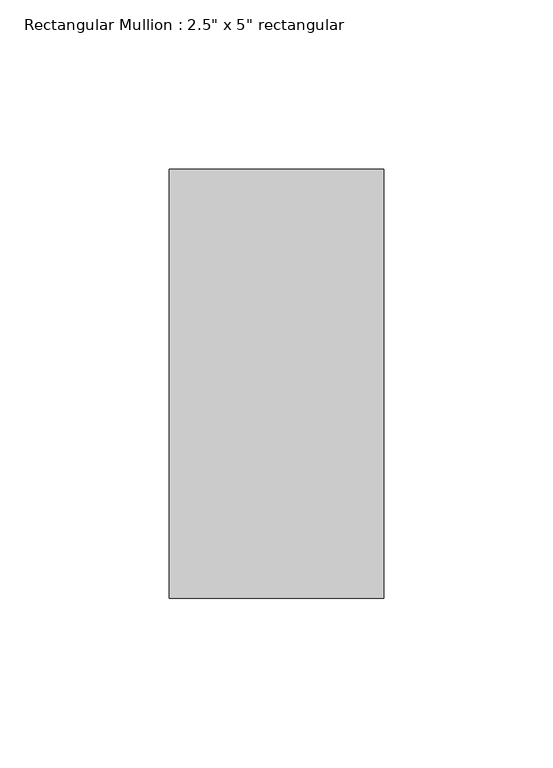
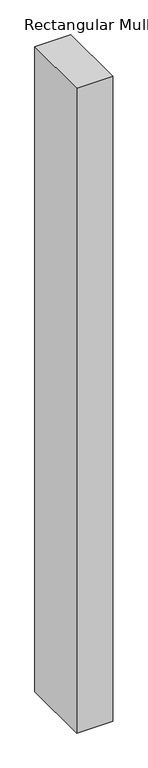
"""IFC4 building model written with IfcOpenShell, lengths in millimetres: member geometry."""

from ifc_helpers import new_model, si_unit, frame, origin, place, context, project, spatial, polyline, outline, extrude, source, transform, mapped, element, save


def member_34ede31c(model_context):
    return source(origin(), model_context, "Body", "SweptSolid", [
        extrude(outline(polyline([(31.75, 63.5), (31.75, -63.5), (-31.75, -63.5), (-31.75, 63.5), (31.75, 63.5)])), frame((0.0, 0.0, -1200.1500001), z_axis=(0.0, 0.0, 1.0), x_axis=(1.0, 0.0, 0.0)), (0.0, 0.0, 1.0), 1200.1500001),
    ])


if __name__ == "__main__":
    model = new_model("IFC4")
    model_context = context("Model", 3, world=origin())
    ifc_project = project(units=[si_unit("LENGTHUNIT", "METRE", prefix="MILLI")], contexts=[model_context])
    site = spatial("IfcSite", under=ifc_project)
    building = spatial("IfcBuilding", under=site)
    placement = place(None, origin())
    member_shape = member_34ede31c(model_context)
    element("IfcMember", 1, ObjectType="Rectangular Mullion : 2.5\" x 5\" rectangular", at=placement, inside=building, context=model_context, shape_type="MappedRepresentation", body=[
        mapped(member_shape, transform((0.0, 0.0, 0.0), x_axis=(1.0, 0.0, 0.0), y_axis=(0.0, 1.0, 0.0), z_axis=(0.0, 0.0, 1.0))),
    ])
    save(model, "model.ifc")

# Revit data of these elements
# Type "Rectangular Mullion : 2.5\" x 5\" rectangular"
#   built-in parameter 1007304 = 0.416667 (stored number, unit not read)
#   built-in parameter 1007301 = 0.104167 (stored number, unit not read)
#   built-in parameter 1007300 = 0.104167 (stored number, unit not read)
# Element 1 (IfcMember, "Rectangular Mullion : 2.5\" x 5\" rectangular")
#   Materials on its faces: "Aluminum"
# Materials
#   "Aluminum": class "Metal", colour RGB 247 247 247, transparency 0, Description = "Aluminum 6061", Cost = 0
